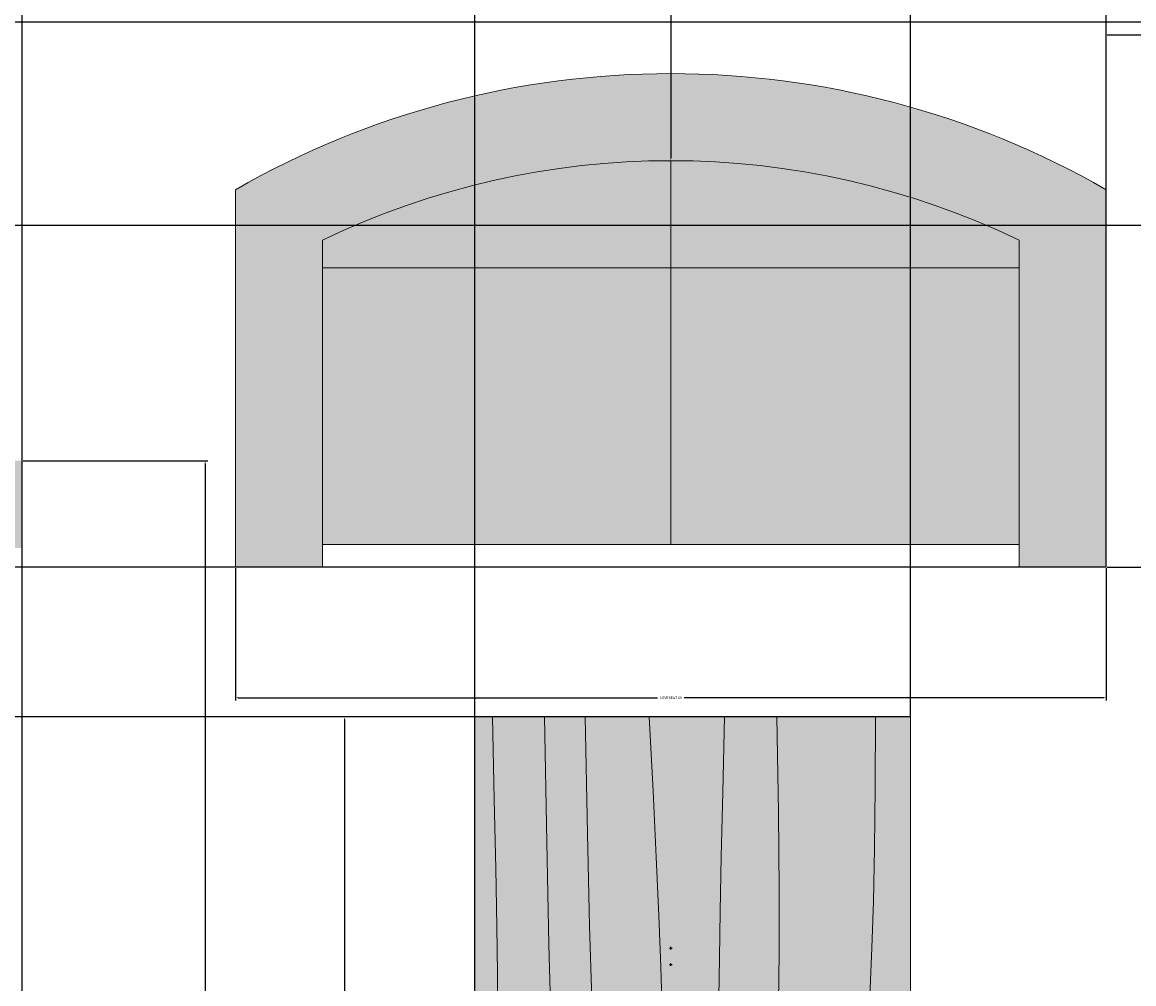
# Model space of a CAD drawing. Units: inches. Extents: x 1201 to 1754, y 247 to 775.
# Tile 4 of 10: x 1305 to 1382, y 491 to 557. Entities that reach past the tile are written whole.
import ezdxf

# ---------------------------------------------------------------- set-up
doc = ezdxf.new("R2010")
doc.units = ezdxf.units.IN
for name, color, linetype, lineweight in [('A-ANNO-DIMS', 2, 'Continuous', 18), ('A-FURN', 8, 'Continuous', 18), ('A-FURN-PATT', 9, 'Continuous', 13)]:
    doc.layers.add(name, color=color, linetype=linetype, lineweight=lineweight)
doc.styles.get("Standard").update_dxf_attribs({"font": 'arial.ttf'})
doc.dimstyles.get("Standard").update_dxf_attribs({"dimtxt": 0.18, "dimasz": 0.18, "dimexe": 0.18, "dimexo": 0.0625, "dimgap": 0.09, "dimtad": 0, "dimtih": 1, "dimtoh": 1, "dimdec": 4, "dimzin": 0, "dimdsep": 46, "dimtxsty": 'Standard', "dimcen": 0.09, "dimadec": 0, "dimazin": 0, "dimtfac": 1, "dimtdec": 4, "dimtofl": 0, "dimtmove": 0, "dimatfit": 3, "dimfxl": 1, "dimtolj": 1, "dimtzin": 0, "dimarcsym": 0})

# ---------------------------------------------------------------- blocks, each defined once
blk = doc.blocks.new('Sofa - Roundback Loveseat 5 ft.')
for p, q in [((0, -32.44198), (0, -5.99998)), ((-24, -33.99998), (-24, -11.46958)), ((24.00004, -33.99998), (24.00004, -11.46958)), ((-23.9998, -13.38178), (23.99986, -13.38178)), ((-24, -32.44198), (24.00004, -32.44198))]:
    blk.add_line(p, q)
for points in [[(-24, -33.99998), (-30, -33.99998), (-30, -7.99998)], [(30.00004, -7.99998), (30.00004, -33.99998), (24.00004, -33.99998)]]:
    blk.add_lwpolyline(points)
for centre, radius, start, end in [((0, -60.24998), 60.24998, 60.13715, 119.8628), ((0, -61.38438), 55.38444, 64.32083, 115.6792)]:
    blk.add_arc(centre, radius, start, end)
blk = doc.blocks.new('Table - Rectangular Woodgrain 60 x 30 in.')
for p, q in [((0, 0), (0, -30)), ((60, 0), (0, 0)), ((60, -30), (60, 0)), ((0, -30), (60, -30))]:
    blk.add_line(p, q)
for points in [[(0, -2.4), (4.8155, -2.418), (9.0302, -2.4688), (12.709, -2.5477), (15.9167, -2.65), (18.7181, -2.7711), (21.1781, -2.9063), (23.3616, -3.0508), (25.3333, -3.2), (27.1477, -3.3495), (28.8172, -3.4958), (30.3437, -3.636), (31.7291, -3.7667), (32.9756, -3.8849), (34.0849, -3.9875), (35.059, -4.0714), (35.9, -4.1334), (36.6114, -4.1711), (37.2041, -4.1854), (37.6906, -4.1779), (38.0833, -4.15), (38.3948, -4.1034), (38.6375, -4.0396), (38.8239, -3.9602), (38.9666, -3.8667), (39.0764, -3.7608), (39.1573, -3.6448), (39.2116, -3.521), (39.2416, -3.3917), (39.2498, -3.2593), (39.2385, -3.1261), (39.21, -2.9944), (39.1666, -2.8667), (39.111, -2.7447), (39.0468, -2.6281), (38.978, -2.5163), (38.9083, -2.4083), (38.8418, -2.3035), (38.7823, -2.201), (38.7337, -2.1001), (38.7, -2), (38.6844, -1.9003), (38.6875, -1.8021), (38.7094, -1.707), (38.75, -1.6167), (38.8094, -1.5326), (38.8875, -1.4563), (38.9844, -1.3893), (39.1, -1.3333), (39.2351, -1.2896), (39.3937, -1.2583), (39.5804, -1.2396), (39.8, -1.2333), (40.057, -1.2396), (40.3562, -1.2583), (40.7023, -1.2896), (41.1, -1.3333), (41.5547, -1.3895), (42.0755, -1.4573), (42.6721, -1.5361), (43.3542, -1.625), (44.1316, -1.7233), (45.014, -1.8302), (46.0114, -1.9449), (47.1333, -2.0667), (48.3862, -2.1947), (49.7625, -2.3281), (51.2513, -2.4663), (52.8416, -2.6083), (54.5226, -2.7535), (56.2833, -2.9011), (58.1127, -3.0501), (60, -3.2)], [(0, -9.2), (6.5759, -9.0858), (11.9385, -9.0365), (16.2527, -9.0418), (19.6833, -9.0917), (22.3952, -9.1759), (24.5531, -9.2844), (26.322, -9.4069), (27.8666, -9.5333), (29.3241, -9.6553), (30.7203, -9.7719), (32.0532, -9.8837), (33.3208, -9.9917), (34.5213, -10.0965), (35.6526, -10.199), (36.7128, -10.2999), (37.7, -10.4), (38.6129, -10.4996), (39.4531, -10.5969), (40.223, -10.6895), (40.925, -10.775), (41.5613, -10.8512), (42.1344, -10.9156), (42.6465, -10.966), (43.1, -11), (43.4976, -11.0158), (43.8437, -11.0136), (44.143, -10.9942), (44.4, -10.9583), (44.6195, -10.9069), (44.8062, -10.8406), (44.9648, -10.7603), (45.1, -10.6667), (45.2155, -10.5598), (45.3114, -10.4365), (45.3871, -10.2929), (45.4416, -10.125), (45.4743, -9.929), (45.4844, -9.7011), (45.4709, -9.4371), (45.4333, -9.1333), (45.3716, -8.7883), (45.2896, -8.4104), (45.1919, -8.0107), (45.0833, -7.6), (44.9685, -7.1893), (44.8521, -6.7896), (44.7388, -6.4117), (44.6333, -6.0667), (44.54, -5.7628), (44.4614, -5.4979), (44.4001, -5.2675), (44.3583, -5.0667), (44.3384, -4.8909), (44.3427, -4.7354), (44.3736, -4.5956), (44.4333, -4.4667), (44.5236, -4.3453), (44.6427, -4.2333), (44.7884, -4.1339), (44.9583, -4.05), (45.1501, -3.9849), (45.3614, -3.9417), (45.59, -3.9234), (45.8333, -3.9333), (46.0915, -3.9749), (46.3734, -4.0531), (46.6906, -4.1736), (47.0542, -4.3417), (47.4756, -4.5629), (47.9661, -4.8427), (48.5372, -5.1866), (49.2, -5.6), (49.9676, -6.0844), (50.8594, -6.625), (51.8965, -7.2031), (53.1, -7.8), (54.491, -8.3969), (56.0906, -8.975), (57.9199, -9.5156), (60, -10)], [(0, -12.8), (5.1847, -12.9322), (9.6213, -13.0323), (13.3963, -13.1059), (16.5958, -13.1583), (19.3063, -13.1952), (21.614, -13.2219), (23.6054, -13.2439), (25.3666, -13.2667), (26.9728, -13.2947), (28.4531, -13.3281), (29.8256, -13.3663), (31.1083, -13.4083), (32.3191, -13.4535), (33.476, -13.501), (34.597, -13.5501), (35.7, -13.6), (36.7984, -13.6497), (37.8875, -13.6979), (38.9578, -13.743), (40, -13.7833), (41.0047, -13.8174), (41.9625, -13.8438), (42.864, -13.8607), (43.7, -13.8667), (44.4631, -13.8604), (45.1552, -13.8417), (45.7801, -13.8104), (46.3416, -13.7667), (46.8439, -13.7104), (47.2906, -13.6417), (47.6858, -13.5604), (48.0333, -13.4667), (48.3375, -13.3608), (48.6042, -13.2448), (48.8396, -13.121), (49.05, -12.9917), (49.2417, -12.8593), (49.4208, -12.7261), (49.5937, -12.5944), (49.7667, -12.4667), (49.9452, -12.3451), (50.1323, -12.2313), (50.3303, -12.1268), (50.5416, -12.0333), (50.7686, -11.9524), (51.0135, -11.8854), (51.2788, -11.8341), (51.5666, -11.8), (51.8785, -11.7843), (52.2116, -11.7865), (52.562, -11.8059), (52.926, -11.8417), (53.2998, -11.8931), (53.6795, -11.9594), (54.0614, -12.0397), (54.4416, -12.1333), (54.8223, -12.2401), (55.2293, -12.3625), (55.6942, -12.5037), (56.2489, -12.6667), (56.9251, -12.8547), (57.7545, -13.0708), (58.7689, -13.3182), (60, -13.6)], [(0, -18), (5.124, -17.7273), (9.6609, -17.5057), (13.6705, -17.3303), (17.2125, -17.1958), (20.3467, -17.0973), (23.1328, -17.0297), (25.6307, -16.9878), (27.9, -16.9667), (29.9928, -16.9617), (31.9302, -16.9703), (33.7254, -16.9907), (35.3917, -17.0208), (36.9423, -17.0588), (38.3906, -17.1026), (39.7499, -17.1503), (41.0333, -17.2), (42.2519, -17.2496), (43.4073, -17.2969), (44.4986, -17.3395), (45.525, -17.375), (46.4858, -17.4012), (47.3802, -17.4156), (48.2074, -17.416), (48.9667, -17.4), (49.6583, -17.3662), (50.2872, -17.3167), (50.8595, -17.2547), (51.3812, -17.1833), (51.8584, -17.1057), (52.2971, -17.025), (52.7034, -16.9443), (53.0833, -16.8667), (53.443, -16.7951), (53.789, -16.7313), (54.128, -16.6768), (54.4666, -16.6334), (54.8115, -16.6024), (55.1693, -16.5854), (55.5465, -16.5841), (55.95, -16.6), (56.3828, -16.6337), (56.8346, -16.6823), (57.2915, -16.7418), (57.7396, -16.8084), (58.165, -16.878), (58.5539, -16.9469), (58.8924, -17.0111), (59.1666, -17.0667), (59.3679, -17.1107), (59.5078, -17.1438), (59.6032, -17.1675), (59.6708, -17.1833), (59.7275, -17.193), (59.7901, -17.1979), (59.8753, -17.1998), (60, -17.2)], [(0, -22.4), (8.0098, -22.2501), (14.4094, -22.1011), (19.4168, -21.9535), (23.25, -21.8083), (26.1269, -21.6663), (28.2656, -21.5281), (29.884, -21.3947), (31.2, -21.2667), (32.3967, -21.1448), (33.5172, -21.0292), (34.5697, -20.9198), (35.5625, -20.8167), (36.5037, -20.7198), (37.4015, -20.6292), (38.2642, -20.5448), (39.1, -20.4667), (39.9164, -20.3951), (40.7187, -20.3313), (41.5117, -20.2768), (42.3, -20.2333), (43.0883, -20.2024), (43.8812, -20.1854), (44.6836, -20.1841), (45.5, -20.2), (46.3328, -20.234), (47.1747, -20.2844), (48.0163, -20.3488), (48.8479, -20.425), (49.66, -20.5106), (50.4429, -20.6031), (51.1872, -20.7004), (51.8833, -20.8), (52.5246, -20.8999), (53.1166, -20.9995), (53.6681, -21.0983), (54.1875, -21.1958), (54.6834, -21.2919), (55.1646, -21.3859), (55.6394, -21.4777), (56.1167, -21.5667), (56.6028, -21.6515), (57.0961, -21.7266), (57.5929, -21.7852), (58.0896, -21.8208), (58.5823, -21.8268), (59.0674, -21.7964), (59.5412, -21.723), (60, -21.6)], [(0, -25.2), (8.6355, -25.0504), (15.7026, -24.9031), (21.4049, -24.7606), (25.9458, -24.625), (29.529, -24.4988), (32.3578, -24.3844), (34.6359, -24.284), (36.5667, -24.2), (38.3213, -24.1341), (39.9417, -24.0854), (41.437, -24.0523), (42.8167, -24.0333), (44.0901, -24.0268), (45.2667, -24.0313), (46.3557, -24.0451), (47.3667, -24.0667), (48.309, -24.0947), (49.1928, -24.1287), (50.0284, -24.168), (50.826, -24.2125), (51.5959, -24.2617), (52.3483, -24.3151), (53.0935, -24.3725), (53.8417, -24.4334), (54.6009, -24.497), (55.3699, -24.561), (56.1454, -24.6226), (56.9239, -24.6792), (57.7021, -24.7279), (58.4764, -24.7662), (59.2435, -24.7911), (60, -24.8)], [(0, -28.8), (5.6867, -28.6681), (10.45, -28.5698), (14.407, -28.5012), (17.675, -28.4584), (20.3711, -28.4374), (22.6125, -28.4344), (24.5164, -28.4455), (26.2, -28.4667), (27.762, -28.4947), (29.2276, -28.5281), (30.6033, -28.5663), (31.8958, -28.6084), (33.1118, -28.6535), (34.2578, -28.7011), (35.3405, -28.7501), (36.3666, -28.8), (37.3443, -28.8497), (38.288, -28.8974), (39.2137, -28.9412), (40.1375, -28.9792), (41.0753, -29.0093), (42.0432, -29.0297), (43.0572, -29.0384), (44.1333, -29.0333), (45.2936, -29.0114), (46.5843, -28.9641), (48.0579, -28.8816), (49.7666, -28.7542), (51.7629, -28.5721), (54.0989, -28.3255), (56.8272, -28.0048), (60, -27.6)]]:
    blk.add_lwpolyline(points)
blk = doc.blocks.new('*D31')
at = {"layer": 'A-ANNO-DIMS', "color": 0, "lineweight": -2, "transparency": 16777216}
for p, q in [((1319.706, 519.841), (1319.706, 510.723)), ((1379.706, 519.841), (1379.706, 510.723)), ((1319.886, 510.903), (1348.792, 510.903)), ((1379.526, 510.903), (1350.619, 510.903))]:
    blk.add_line(p, q, dxfattribs=at)
at = {"layer": 'A-ANNO-DIMS', "color": 0, "transparency": 16777216}
for points in [[(1319.886, 510.933), (1319.886, 510.873), (1319.706, 510.903)], [(1379.526, 510.933), (1379.526, 510.873), (1379.706, 510.903)]]:
    blk.add_solid(points, dxfattribs=at)
at = {"layer": 'Defpoints', "color": 0, "transparency": 16777216}
for p in [(1319.706, 519.903), (1379.706, 519.903), (1379.706, 510.903)]:
    blk.add_point(p, dxfattribs=at)
at = {"layer": 'A-ANNO-DIMS', "color": 0, "transparency": 16777216, "insert": (1349.706, 510.903), "char_height": 0.18, "attachment_point": 5}
blk.add_mtext('\\A1;LOVESEAT 60', dxfattribs=at)
blk = doc.blocks.new('*D32')
at = {"layer": 'A-ANNO-DIMS', "color": 0, "lineweight": -2, "transparency": 16777216}
for p, q in [((1379.768, 556.57), (1388.886, 556.57)), ((1388.706, 556.39), (1388.706, 538.419)), ((1388.706, 520.083), (1388.706, 538.055)), ((1379.768, 519.903), (1388.886, 519.903))]:
    blk.add_line(p, q, dxfattribs=at)
at = {"layer": 'A-ANNO-DIMS', "color": 0, "transparency": 16777216}
for points in [[(1388.676, 556.39), (1388.736, 556.39), (1388.706, 556.57)], [(1388.676, 520.083), (1388.736, 520.083), (1388.706, 519.903)]]:
    blk.add_solid(points, dxfattribs=at)
at = {"layer": 'Defpoints', "color": 0, "transparency": 16777216}
for p in [(1379.706, 556.57), (1388.706, 556.57), (1379.706, 519.903)]:
    blk.add_point(p, dxfattribs=at)
at = {"layer": 'A-ANNO-DIMS', "color": 0, "transparency": 16777216, "insert": (1388.706, 538.237), "char_height": 0.18, "attachment_point": 5}
blk.add_mtext('\\A1;37', dxfattribs=at)
blk = doc.blocks.new('*D35')
at = {"layer": 'A-ANNO-DIMS', "color": 0, "lineweight": -2, "transparency": 16777216}
for p, q in [((1336.149, 509.584), (1327.031, 509.584)), ((1327.211, 509.404), (1327.211, 479.767)), ((1327.211, 449.764), (1327.211, 479.401)), ((1336.149, 449.584), (1327.031, 449.584))]:
    blk.add_line(p, q, dxfattribs=at)
at = {"layer": 'A-ANNO-DIMS', "color": 0, "transparency": 16777216}
for points in [[(1327.181, 509.404), (1327.241, 509.404), (1327.211, 509.584)], [(1327.181, 449.764), (1327.241, 449.764), (1327.211, 449.584)]]:
    blk.add_solid(points, dxfattribs=at)
at = {"layer": 'Defpoints', "color": 0, "transparency": 16777216}
for p in [(1336.211, 509.584), (1327.211, 449.584), (1336.211, 449.584)]:
    blk.add_point(p, dxfattribs=at)
at = {"layer": 'A-ANNO-DIMS', "color": 0, "transparency": 16777216, "insert": (1327.211, 479.584), "char_height": 0.18, "attachment_point": 5}
blk.add_mtext('\\A1;COFFEE TABLE 60', dxfattribs=at)
blk = doc.blocks.new('*D37')
at = {"layer": 'A-ANNO-DIMS', "color": 0, "lineweight": -2, "transparency": 16777216}
for p, q in [((1305.079, 527.227), (1317.797, 527.227)), ((1317.617, 527.047), (1317.617, 485.41)), ((1317.617, 443.407), (1317.617, 485.044)), ((1305.079, 443.227), (1317.797, 443.227))]:
    blk.add_line(p, q, dxfattribs=at)
at = {"layer": 'A-ANNO-DIMS', "color": 0, "transparency": 16777216}
for points in [[(1317.587, 527.047), (1317.647, 527.047), (1317.617, 527.227)], [(1317.587, 443.407), (1317.647, 443.407), (1317.617, 443.227)]]:
    blk.add_solid(points, dxfattribs=at)
at = {"layer": 'Defpoints', "color": 0, "transparency": 16777216}
for p in [(1305.017, 527.227), (1317.617, 527.227), (1305.017, 443.227)]:
    blk.add_point(p, dxfattribs=at)
at = {"layer": 'A-ANNO-DIMS', "color": 0, "transparency": 16777216, "insert": (1317.617, 485.227), "char_height": 0.18, "attachment_point": 5}
blk.add_mtext('\\A1;SOFA 84', dxfattribs=at)
blk = doc.blocks.new('*D59')
at = {"layer": 'A-ANNO-DIMS', "color": 0, "lineweight": -2, "transparency": 16777216}
for p, q in [((1255.521, 418.004), (1255.521, 775.136)), ((1405.521, 418.004), (1405.521, 775.136)), ((1255.701, 774.956), (1330.241, 774.956)), ((1405.341, 774.956), (1330.801, 774.956))]:
    blk.add_line(p, q, dxfattribs=at)
at = {"layer": 'A-ANNO-DIMS', "color": 0, "transparency": 16777216}
for points in [[(1255.701, 774.986), (1255.701, 774.926), (1255.521, 774.956)], [(1405.341, 774.986), (1405.341, 774.926), (1405.521, 774.956)]]:
    blk.add_solid(points, dxfattribs=at)
at = {"layer": 'Defpoints', "color": 0, "transparency": 16777216}
for p in [(1405.521, 774.956), (1255.521, 417.941), (1405.521, 417.941)]:
    blk.add_point(p, dxfattribs=at)
at = {"layer": 'A-ANNO-DIMS', "color": 0, "transparency": 16777216, "insert": (1330.521, 774.956), "char_height": 0.18, "attachment_point": 5}
blk.add_mtext('\\A1;150', dxfattribs=at)
blk = doc.blocks.new('*D75')
at = {"layer": 'A-ANNO-DIMS', "color": 0, "lineweight": -2, "transparency": 16777216}
for p, q in [((1717.458, 557.441), (1222.326, 557.441)), ((1222.506, 557.261), (1222.506, 550.621)), ((1222.506, 543.616), (1222.506, 550.257)), ((1717.458, 543.436), (1222.326, 543.436))]:
    blk.add_line(p, q, dxfattribs=at)
at = {"layer": 'A-ANNO-DIMS', "color": 0, "transparency": 16777216}
for points in [[(1222.476, 557.261), (1222.536, 557.261), (1222.506, 557.441)], [(1222.476, 543.616), (1222.536, 543.616), (1222.506, 543.436)]]:
    blk.add_solid(points, dxfattribs=at)
at = {"layer": 'Defpoints', "color": 0, "transparency": 16777216}
for p in [(1222.506, 557.441), (1717.521, 557.441), (1717.521, 543.436)]:
    blk.add_point(p, dxfattribs=at)
at = {"layer": 'A-ANNO-DIMS', "color": 0, "transparency": 16777216, "insert": (1222.506, 550.439), "char_height": 0.18, "attachment_point": 5}
blk.add_mtext('\\A1;14.005', dxfattribs=at)
blk = doc.blocks.new('*D83')
at = {"layer": 'A-ANNO-DIMS', "color": 0, "lineweight": -2, "transparency": 16777216}
for p, q in [((1471.458, 561.969), (1222.326, 561.969)), ((1222.506, 561.789), (1222.506, 559.887)), ((1222.506, 557.621), (1222.506, 559.523)), ((1471.458, 557.441), (1222.326, 557.441))]:
    blk.add_line(p, q, dxfattribs=at)
at = {"layer": 'A-ANNO-DIMS', "color": 0, "transparency": 16777216}
for points in [[(1222.476, 561.789), (1222.536, 561.789), (1222.506, 561.969)], [(1222.476, 557.621), (1222.536, 557.621), (1222.506, 557.441)]]:
    blk.add_solid(points, dxfattribs=at)
at = {"layer": 'Defpoints', "color": 0, "transparency": 16777216}
for p in [(1222.506, 561.969), (1471.521, 561.969), (1471.521, 557.441)]:
    blk.add_point(p, dxfattribs=at)
at = {"layer": 'A-ANNO-DIMS', "color": 0, "transparency": 16777216, "insert": (1222.506, 559.705), "char_height": 0.18, "attachment_point": 5}
blk.add_mtext('\\A1;4.528', dxfattribs=at)
blk = doc.blocks.new('*D94')
at = {"layer": 'A-ANNO-DIMS', "color": 0, "lineweight": -2, "transparency": 16777216}
for p, q in [((1305.017, 443.289), (1305.017, 775.136)), ((1336.211, 449.646), (1336.211, 775.136)), ((1305.197, 774.956), (1320.15, 774.956)), ((1336.031, 774.956), (1321.078, 774.956))]:
    blk.add_line(p, q, dxfattribs=at)
at = {"layer": 'A-ANNO-DIMS', "color": 0, "transparency": 16777216}
for points in [[(1305.197, 774.986), (1305.197, 774.926), (1305.017, 774.956)], [(1336.031, 774.986), (1336.031, 774.926), (1336.211, 774.956)]]:
    blk.add_solid(points, dxfattribs=at)
at = {"layer": 'Defpoints', "color": 0, "transparency": 16777216}
for p in [(1336.211, 774.956), (1336.211, 449.584), (1305.017, 443.227)]:
    blk.add_point(p, dxfattribs=at)
at = {"layer": 'A-ANNO-DIMS', "color": 0, "transparency": 16777216, "insert": (1320.614, 774.956), "char_height": 0.18, "attachment_point": 5}
blk.add_mtext('\\A1;31.195', dxfattribs=at)
blk = doc.blocks.new('*D98')
at = {"layer": 'A-ANNO-DIMS', "color": 0, "lineweight": -2, "transparency": 16777216}
for p, q in [((1366.211, 509.646), (1366.211, 775.136)), ((1379.706, 519.966), (1379.706, 775.136)), ((1366.391, 774.956), (1372.504, 774.956)), ((1379.526, 774.956), (1373.413, 774.956))]:
    blk.add_line(p, q, dxfattribs=at)
at = {"layer": 'A-ANNO-DIMS', "color": 0, "transparency": 16777216}
for points in [[(1366.391, 774.986), (1366.391, 774.926), (1366.211, 774.956)], [(1379.526, 774.986), (1379.526, 774.926), (1379.706, 774.956)]]:
    blk.add_solid(points, dxfattribs=at)
at = {"layer": 'Defpoints', "color": 0, "transparency": 16777216}
for p in [(1379.706, 774.956), (1379.706, 519.903), (1366.211, 509.584)]:
    blk.add_point(p, dxfattribs=at)
at = {"layer": 'A-ANNO-DIMS', "color": 0, "transparency": 16777216, "insert": (1372.959, 774.956), "char_height": 0.18, "attachment_point": 5}
blk.add_mtext('\\A1;13.494', dxfattribs=at)
blk = doc.blocks.new('*D99')
at = {"layer": 'A-ANNO-DIMS', "color": 0, "lineweight": -2, "transparency": 16777216}
for p, q in [((1379.643, 519.903), (1222.326, 519.903)), ((1222.506, 519.723), (1222.506, 514.926)), ((1222.506, 509.764), (1222.506, 514.562)), ((1366.149, 509.584), (1222.326, 509.584))]:
    blk.add_line(p, q, dxfattribs=at)
at = {"layer": 'A-ANNO-DIMS', "color": 0, "transparency": 16777216}
for points in [[(1222.476, 519.723), (1222.536, 519.723), (1222.506, 519.903)], [(1222.476, 509.764), (1222.536, 509.764), (1222.506, 509.584)]]:
    blk.add_solid(points, dxfattribs=at)
at = {"layer": 'Defpoints', "color": 0, "transparency": 16777216}
for p in [(1222.506, 519.903), (1379.706, 519.903), (1366.211, 509.584)]:
    blk.add_point(p, dxfattribs=at)
at = {"layer": 'A-ANNO-DIMS', "color": 0, "transparency": 16777216, "insert": (1222.506, 514.744), "char_height": 0.18, "attachment_point": 5}
blk.add_mtext('\\A1;10.32', dxfattribs=at)
blk = doc.blocks.new('*D103')
at = {"layer": 'A-ANNO-DIMS', "color": 0, "lineweight": -2, "transparency": 16777216}
for p, q in [((1349.886, 590.053), (1349.706, 590.053)), ((1349.706, 590.053), (1349.706, 554.083)), ((1349.616, 493.653), (1349.796, 493.653)), ((1349.706, 493.563), (1349.706, 493.743))]:
    blk.add_line(p, q, dxfattribs=at)
at = {"layer": 'A-ANNO-DIMS', "color": 0, "transparency": 16777216}
blk.add_solid([(1349.676, 554.083), (1349.736, 554.083), (1349.706, 553.903)], dxfattribs=at)
at = {"layer": 'Defpoints', "color": 0, "transparency": 16777216}
for p in [(1349.706, 553.903), (1349.706, 493.653)]:
    blk.add_point(p, dxfattribs=at)
at = {"layer": 'A-ANNO-DIMS', "color": 0, "transparency": 16777216, "insert": (1350.367, 590.053), "char_height": 0.18, "attachment_point": 5}
blk.add_mtext('\\A1;R60.25', dxfattribs=at)
blk = doc.blocks.new('*D104')
at = {"layer": 'A-ANNO-DIMS', "color": 0, "lineweight": -2, "transparency": 16777216}
for p, q in [((1349.886, 581.134), (1349.706, 581.134)), ((1349.706, 581.134), (1349.706, 548.084)), ((1349.616, 492.519), (1349.796, 492.519)), ((1349.706, 492.429), (1349.706, 492.609))]:
    blk.add_line(p, q, dxfattribs=at)
at = {"layer": 'A-ANNO-DIMS', "color": 0, "transparency": 16777216}
blk.add_solid([(1349.676, 548.084), (1349.736, 548.084), (1349.706, 547.904)], dxfattribs=at)
at = {"layer": 'Defpoints', "color": 0, "transparency": 16777216}
for p in [(1349.706, 547.904), (1349.706, 492.519)]:
    blk.add_point(p, dxfattribs=at)
at = {"layer": 'A-ANNO-DIMS', "color": 0, "transparency": 16777216, "insert": (1350.366, 581.134), "char_height": 0.18, "attachment_point": 5}
blk.add_mtext('\\A1;R55.38', dxfattribs=at)

msp = doc.modelspace()

# ---------------------------------------------------------------- hatches: boundary and pattern name
at = {"layer": 'A-FURN-PATT'}
h = msp.add_hatch(color=256, dxfattribs=at)
h.dxf.hatch_style = 1
h.paths.add_polyline_path([(1373.7057, 540.5217), (1349.7056, 540.5217), (1349.7056, 521.4615), (1373.7057, 521.4615)], flags=17)
h.paths.add_polyline_path([(1349.7056, 540.5217), (1325.7056, 540.5217), (1325.7056, 521.4615), (1349.7056, 521.4615)], flags=17)
h.paths.add_polyline_path([(1349.7056, 547.9035, 0.1125187), (1325.7056, 542.4334), (1325.7056, 540.5217), (1349.7056, 540.5217)], flags=17)
h.paths.add_polyline_path([(1349.7056, 547.9035), (1349.7056, 540.5217), (1373.7057, 540.5217), (1373.7057, 542.4333, 0.1125189)], flags=17)
h.paths.add_polyline_path([(1319.7056, 545.9034), (1319.7056, 519.9035), (1325.7056, 519.9035), (1325.7056, 542.4334, -0.2279232), (1373.7057, 542.4333), (1373.7057, 540.5217), (1373.7057, 521.4615), (1373.7057, 519.9035), (1379.7057, 519.9035), (1379.7057, 545.9034, 0.266667)])
h.paths.add_polyline_path([(1303.4586, 521.2267), (1284.3984, 521.2267), (1284.3984, 497.2267), (1303.4586, 497.2267)], flags=17)
h.paths.add_polyline_path([(1303.4586, 497.2267), (1284.3984, 497.2267), (1284.3984, 473.2267), (1303.4586, 473.2267)], flags=17)
h.paths.add_polyline_path([(1303.4586, 473.2267), (1284.3984, 473.2267), (1284.3984, 449.2267), (1303.4586, 449.2267)], flags=17)
h.paths.add_polyline_path([(1282.4866, 521.2267), (1305.0165, 521.2267), (1305.0165, 527.2267), (1279.0165, 527.2267, 0.1904762), (1279.0165, 443.2267), (1305.0165, 443.2267), (1305.0165, 449.2267), (1282.4866, 449.2267, -0.1519478)])
h.paths.add_polyline_path([(1284.3984, 497.2267), (1277.612, 497.2267, 0.0496282), (1277.612, 473.2267), (1284.3984, 473.2267)], flags=17)
h.paths.add_polyline_path([(1284.3984, 521.2267), (1282.4866, 521.2267, 0.0506467), (1277.612, 497.2267), (1284.3984, 497.2267)], flags=17)
h.paths.add_polyline_path([(1284.3984, 473.2267), (1277.612, 473.2267, 0.0506466), (1282.4866, 449.2267), (1284.3984, 449.2267)], flags=17)
h = msp.add_hatch(color=256, dxfattribs=at)
h.dxf.hatch_style = 1
h.paths.add_polyline_path([(1363.7933, 504.7684), (1363.8113, 509.5839), (1357.0113, 509.5839), (1357.1255, 503.008), (1357.1748, 497.6454), (1357.1695, 493.3312), (1357.1196, 489.9006), (1357.0354, 487.1887), (1356.9269, 485.0308), (1356.8044, 483.2619), (1356.678, 481.7173), (1356.556, 480.2598), (1356.4394, 478.8636), (1356.3276, 477.5307), (1356.2196, 476.2631), (1356.1148, 475.0626), (1356.0123, 473.9313), (1355.9114, 472.8711), (1355.8113, 471.8839), (1355.7117, 470.971), (1355.6144, 470.1308), (1355.5218, 469.3609), (1355.4363, 468.6589), (1355.3601, 468.0226), (1355.2957, 467.4495), (1355.2453, 466.9374), (1355.2113, 466.4839), (1355.1955, 466.0863), (1355.1977, 465.7402), (1355.2171, 465.4409), (1355.253, 465.1839), (1355.3044, 464.9644), (1355.3707, 464.7777), (1355.451, 464.6191), (1355.5446, 464.4839), (1355.6515, 464.3684), (1355.7748, 464.2725), (1355.9184, 464.1968), (1356.0863, 464.1423), (1356.2823, 464.1096), (1356.5102, 464.0995), (1356.7742, 464.113), (1357.078, 464.1506), (1357.423, 464.2123), (1357.8009, 464.2943), (1358.2006, 464.392), (1358.6113, 464.5006), (1359.022, 464.6154), (1359.4217, 464.7318), (1359.7996, 464.8451), (1360.1446, 464.9506), (1360.4485, 465.0439), (1360.7134, 465.1225), (1360.9438, 465.1838), (1361.1446, 465.2256), (1361.3204, 465.2455), (1361.4759, 465.2412), (1361.6157, 465.2103), (1361.7446, 465.1506), (1361.866, 465.0603), (1361.978, 464.9412), (1362.0774, 464.7955), (1362.1613, 464.6256), (1362.2264, 464.4338), (1362.2696, 464.2225), (1362.2879, 463.9939), (1362.278, 463.7506), (1362.2364, 463.4924), (1362.1582, 463.2105), (1362.0377, 462.8933), (1361.8696, 462.5297), (1361.6484, 462.1083), (1361.3686, 461.6178), (1361.0247, 461.0467), (1360.6113, 460.3839), (1360.1269, 459.6163), (1359.5863, 458.7245), (1359.0082, 457.6874), (1358.4113, 456.4839), (1357.8144, 455.0929), (1357.2363, 453.4933), (1356.6957, 451.664), (1356.2113, 449.5839), (1363.0113, 449.5839), (1363.1612, 451.4712), (1363.3102, 453.3006), (1363.4578, 455.0613), (1363.603, 456.7423), (1363.745, 458.3326), (1363.8832, 459.8214), (1364.0166, 461.1977), (1364.1446, 462.4506), (1364.2664, 463.5725), (1364.3811, 464.5699), (1364.488, 465.4523), (1364.5863, 466.2297), (1364.6752, 466.9118), (1364.754, 467.5084), (1364.8218, 468.0292), (1364.878, 468.4839), (1364.9217, 468.8816), (1364.953, 469.2277), (1364.9717, 469.5269), (1364.978, 469.7839), (1364.9717, 470.0035), (1364.953, 470.1902), (1364.9217, 470.3488), (1364.878, 470.4839), (1364.822, 470.5995), (1364.755, 470.6964), (1364.6787, 470.7745), (1364.5946, 470.8339), (1364.5043, 470.8745), (1364.4092, 470.8964), (1364.311, 470.8995), (1364.2113, 470.8839), (1364.1112, 470.8502), (1364.0103, 470.8016), (1363.9078, 470.7421), (1363.803, 470.6756), (1363.6186, 470.5566), (1363.3995, 470.436), (1363.149, 470.3508), (1362.881, 470.3281), (1362.6903, 470.3723), (1362.5665, 470.4266), (1362.4505, 470.5075), (1362.3446, 470.6173), (1362.2511, 470.76), (1362.1717, 470.9464), (1362.1079, 471.1891), (1362.0613, 471.5006), (1362.0334, 471.8933), (1362.0259, 472.3798), (1362.0402, 472.9725), (1362.0779, 473.6839), (1362.1399, 474.5249), (1362.2238, 475.499), (1362.3264, 476.6083), (1362.4446, 477.8548), (1362.5753, 479.2402), (1362.7155, 480.7667), (1362.8618, 482.4362), (1363.0113, 484.2506), (1363.1605, 486.2223), (1363.305, 488.4058), (1363.4402, 490.8658), (1363.5613, 493.6672), (1363.6636, 496.8749), (1363.7425, 500.5537)])
h.paths.add_polyline_path([(1342.1259, 469.6422), (1342.0772, 471.2626), (1342.0113, 473.0172), (1341.9273, 474.948), (1341.8269, 477.2261), (1341.7125, 480.0549), (1341.5863, 483.6381), (1341.4507, 488.179), (1341.3082, 493.8813), (1341.1609, 500.9484), (1341.0113, 509.5839), (1337.4113, 509.5839), (1337.5432, 503.8972), (1337.6415, 499.1339), (1337.7101, 495.1769), (1337.7529, 491.9089), (1337.7739, 489.2128), (1337.7769, 486.9714), (1337.7658, 485.0675), (1337.7446, 483.3839), (1337.7166, 481.8219), (1337.6832, 480.3563), (1337.645, 478.9806), (1337.6029, 477.6881), (1337.5578, 476.4721), (1337.5102, 475.3261), (1337.4612, 474.2434), (1337.4113, 473.2173), (1337.3616, 472.2396), (1337.3139, 471.2959), (1337.2701, 470.3702), (1337.2321, 469.4464), (1337.202, 468.5086), (1337.1816, 467.5407), (1337.1729, 466.5267), (1337.178, 465.4506), (1337.1999, 464.2903), (1337.2472, 462.9996), (1337.3297, 461.526), (1337.4571, 459.8173), (1337.6392, 457.821), (1337.8858, 455.485), (1338.2065, 452.7567), (1338.6113, 449.5839), (1341.4113, 449.5839), (1341.4202, 450.3404), (1341.4451, 451.1075), (1341.4834, 451.8818), (1341.5321, 452.66), (1341.5887, 453.4385), (1341.6503, 454.214), (1341.7143, 454.983), (1341.7779, 455.7422), (1341.8388, 456.4904), (1341.8962, 457.2356), (1341.9496, 457.988), (1341.9988, 458.7579), (1342.0433, 459.5555), (1342.0826, 460.3911), (1342.1166, 461.2749), (1342.1446, 462.2172), (1342.1662, 463.2282), (1342.18, 464.3172), (1342.1845, 465.4938), (1342.178, 466.7672), (1342.159, 468.1469)])
h.paths.add_polyline_path([(1345.8625, 461.5676), (1345.9269, 462.4092), (1345.9773, 463.2511), (1346.0113, 464.0839), (1346.0272, 464.9003), (1346.0259, 465.7027), (1346.0089, 466.4956), (1345.978, 467.2839), (1345.9345, 468.0722), (1345.88, 468.8652), (1345.8162, 469.6675), (1345.7446, 470.4839), (1345.6665, 471.3197), (1345.5821, 472.1824), (1345.4915, 473.0802), (1345.3946, 474.0214), (1345.2915, 475.0142), (1345.1821, 476.0667), (1345.0665, 477.1872), (1344.9446, 478.3839), (1344.8166, 479.6999), (1344.6832, 481.3183), (1344.545, 483.457), (1344.403, 486.3339), (1344.2578, 490.1671), (1344.1102, 495.1745), (1343.9612, 501.5741), (1343.8113, 509.5839), (1341.0113, 509.5839), (1341.1609, 500.9484), (1341.3082, 493.8813), (1341.4507, 488.179), (1341.5863, 483.6381), (1341.7125, 480.0549), (1341.8269, 477.2261), (1341.9273, 474.948), (1342.0113, 473.0172), (1342.0772, 471.2626), (1342.1259, 469.6422), (1342.159, 468.1469), (1342.178, 466.7672), (1342.1845, 465.4938), (1342.18, 464.3172), (1342.1662, 463.2282), (1342.1446, 462.2172), (1342.1166, 461.2749), (1342.0826, 460.3911), (1342.0433, 459.5555), (1341.9988, 458.7579), (1341.9496, 457.988), (1341.8962, 457.2356), (1341.8388, 456.4904), (1341.7779, 455.7422), (1341.7143, 454.983), (1341.6503, 454.214), (1341.5887, 453.4385), (1341.5321, 452.66), (1341.4834, 451.8818), (1341.4451, 451.1075), (1341.4202, 450.3404), (1341.4113, 449.5839), (1344.6113, 449.5839), (1344.4883, 450.0427), (1344.4149, 450.5165), (1344.3845, 451.0016), (1344.3905, 451.4943), (1344.4261, 451.991), (1344.4847, 452.4878), (1344.5598, 452.9811), (1344.6446, 453.4672), (1344.7336, 453.9445), (1344.8254, 454.4193), (1344.9194, 454.9005), (1345.0155, 455.3964), (1345.113, 455.9158), (1345.2118, 456.4673), (1345.3114, 457.0593), (1345.4113, 457.7006), (1345.5109, 458.3967), (1345.6082, 459.141), (1345.7007, 459.9239), (1345.7863, 460.736)])
h.paths.add_polyline_path([(1349.1056, 457.7255), (1349.028, 458.2027), (1348.9566, 458.7244), (1348.8946, 459.2967), (1348.8451, 459.9256), (1348.8113, 460.6172), (1348.7953, 461.3765), (1348.7957, 462.2037), (1348.8101, 463.0981), (1348.8363, 464.0589), (1348.8718, 465.0853), (1348.9144, 466.1766), (1348.9617, 467.332), (1349.0113, 468.5506), (1349.061, 469.834), (1349.1087, 471.1933), (1349.1525, 472.6416), (1349.1905, 474.1922), (1349.2206, 475.8585), (1349.241, 477.6537), (1349.2496, 479.5911), (1349.2446, 481.6839), (1349.2235, 483.9532), (1349.1816, 486.4511), (1349.114, 489.2372), (1349.0155, 492.3714), (1348.881, 495.9134), (1348.7056, 499.923), (1348.484, 504.4599), (1348.2113, 509.5839), (1343.8113, 509.5839), (1343.9612, 501.5741), (1344.1102, 495.1745), (1344.2578, 490.1671), (1344.403, 486.3339), (1344.545, 483.457), (1344.6832, 481.3183), (1344.8166, 479.6999), (1344.9446, 478.3839), (1345.0665, 477.1872), (1345.1821, 476.0667), (1345.2915, 475.0142), (1345.3946, 474.0214), (1345.4915, 473.0802), (1345.5821, 472.1824), (1345.6665, 471.3197), (1345.7446, 470.4839), (1345.8162, 469.6675), (1345.88, 468.8652), (1345.9345, 468.0722), (1345.978, 467.2839), (1346.0089, 466.4956), (1346.0259, 465.7027), (1346.0272, 464.9003), (1346.0113, 464.0839), (1345.9773, 463.2511), (1345.9269, 462.4092), (1345.8625, 461.5676), (1345.7863, 460.736), (1345.7007, 459.9239), (1345.6082, 459.141), (1345.5109, 458.3967), (1345.4113, 457.7006), (1345.3114, 457.0593), (1345.2118, 456.4673), (1345.113, 455.9158), (1345.0155, 455.3964), (1344.9194, 454.9005), (1344.8254, 454.4193), (1344.7336, 453.9445), (1344.6446, 453.4672), (1344.5598, 452.9811), (1344.4847, 452.4878), (1344.4261, 451.991), (1344.3905, 451.4943), (1344.3845, 451.0016), (1344.4149, 450.5165), (1344.4883, 450.0427), (1344.6113, 449.5839), (1349.0113, 449.5839), (1349.0117, 449.8177), (1349.0302, 449.9259), (1349.0675, 450.0761), (1349.1006, 450.216), (1349.1446, 450.4173), (1349.2002, 450.6915), (1349.2644, 451.03), (1349.3333, 451.4189), (1349.4029, 451.8443), (1349.4695, 452.2924), (1349.529, 452.7493), (1349.5776, 453.2011), (1349.6113, 453.6339), (1349.6272, 454.0374), (1349.6259, 454.4146), (1349.6089, 454.7724), (1349.5779, 455.1173), (1349.5345, 455.4559), (1349.48, 455.7949), (1349.4162, 456.1409), (1349.3446, 456.5006), (1349.267, 456.8805), (1349.1863, 457.2868)])
h.paths.add_polyline_path([(1354.4248, 457.3723), (1354.427, 457.7054), (1354.4113, 458.0173), (1354.3772, 458.3051), (1354.3259, 458.5704), (1354.2589, 458.8153), (1354.178, 459.0423), (1354.0845, 459.2536), (1353.98, 459.4516), (1353.8662, 459.6387), (1353.7446, 459.8172), (1353.6169, 459.9902), (1353.4852, 460.1631), (1353.352, 460.3422), (1353.2196, 460.5339), (1353.0903, 460.7443), (1352.9665, 460.9797), (1352.8505, 461.2464), (1352.7446, 461.5506), (1352.6509, 461.8981), (1352.5696, 462.2933), (1352.5009, 462.74), (1352.4446, 463.2423), (1352.4009, 463.8038), (1352.3696, 464.4287), (1352.3509, 465.1208), (1352.3446, 465.8839), (1352.3506, 466.7199), (1352.3675, 467.6214), (1352.3939, 468.5792), (1352.428, 469.5839), (1352.4683, 470.6261), (1352.5134, 471.6964), (1352.5616, 472.7855), (1352.6113, 473.8839), (1352.6612, 474.9869), (1352.7103, 476.1079), (1352.7578, 477.2648), (1352.803, 478.4756), (1352.845, 479.7583), (1352.8832, 481.1308), (1352.9166, 482.6111), (1352.9446, 484.2173), (1352.9674, 485.9785), (1352.9894, 487.9699), (1353.0161, 490.2776), (1353.053, 492.9881), (1353.1054, 496.1876), (1353.179, 499.9626), (1353.2791, 504.3992), (1353.4113, 509.5839), (1348.2113, 509.5839), (1348.484, 504.4599), (1348.7056, 499.923), (1348.881, 495.9134), (1349.0155, 492.3714), (1349.114, 489.2372), (1349.1816, 486.4511), (1349.2235, 483.9532), (1349.2446, 481.6839), (1349.2496, 479.5911), (1349.241, 477.6537), (1349.2206, 475.8585), (1349.1905, 474.1922), (1349.1525, 472.6416), (1349.1087, 471.1933), (1349.061, 469.834), (1349.0113, 468.5506), (1348.9617, 467.332), (1348.9144, 466.1766), (1348.8718, 465.0853), (1348.8363, 464.0589), (1348.8101, 463.0981), (1348.7957, 462.2037), (1348.7953, 461.3765), (1348.8113, 460.6172), (1348.8451, 459.9256), (1348.8946, 459.2967), (1348.9566, 458.7244), (1349.028, 458.2027), (1349.1056, 457.7255), (1349.1863, 457.2868), (1349.267, 456.8805), (1349.3446, 456.5006), (1349.4162, 456.1409), (1349.48, 455.7949), (1349.5345, 455.4559), (1349.5779, 455.1173), (1349.6089, 454.7724), (1349.6259, 454.4146), (1349.6272, 454.0374), (1349.6113, 453.6339), (1349.5776, 453.2011), (1349.529, 452.7493), (1349.4695, 452.2924), (1349.4029, 451.8443), (1349.3333, 451.4189), (1349.2644, 451.03), (1349.2002, 450.6915), (1349.1446, 450.4173), (1349.1006, 450.216), (1349.0675, 450.0761), (1349.0438, 449.9807), (1349.028, 449.9131), (1349.0183, 449.8564), (1349.0134, 449.7938), (1349.0115, 449.7086), (1349.0113, 449.5839), (1352.6113, 449.5839), (1352.8931, 450.815), (1353.1405, 451.8294), (1353.3566, 452.6588), (1353.5446, 453.335), (1353.7076, 453.8897), (1353.8488, 454.3546), (1353.9712, 454.7616), (1354.078, 455.1423), (1354.1716, 455.5225), (1354.2519, 455.9044), (1354.3182, 456.2841), (1354.3696, 456.6579), (1354.4054, 457.0219)])
h.paths.add_polyline_path([(1360.1269, 459.6163), (1360.6113, 460.3839), (1361.0247, 461.0467), (1361.3686, 461.6178), (1361.6484, 462.1083), (1361.8696, 462.5297), (1362.0377, 462.8933), (1362.1582, 463.2105), (1362.2364, 463.4924), (1362.278, 463.7506), (1362.2879, 463.9939), (1362.2696, 464.2225), (1362.2264, 464.4338), (1362.1613, 464.6256), (1362.0774, 464.7955), (1361.978, 464.9412), (1361.866, 465.0603), (1361.7446, 465.1506), (1361.6157, 465.2103), (1361.4759, 465.2412), (1361.3204, 465.2455), (1361.1446, 465.2256), (1360.9438, 465.1838), (1360.7134, 465.1225), (1360.4485, 465.0439), (1360.1446, 464.9506), (1359.7996, 464.8451), (1359.4217, 464.7318), (1359.022, 464.6154), (1358.6113, 464.5006), (1358.2006, 464.392), (1357.8009, 464.2943), (1357.423, 464.2123), (1357.078, 464.1506), (1356.7742, 464.113), (1356.5102, 464.0995), (1356.2823, 464.1096), (1356.0863, 464.1423), (1355.9184, 464.1968), (1355.7748, 464.2725), (1355.6515, 464.3684), (1355.5446, 464.4839), (1355.451, 464.6191), (1355.3707, 464.7777), (1355.3044, 464.9644), (1355.253, 465.1839), (1355.2171, 465.4409), (1355.1977, 465.7402), (1355.1955, 466.0863), (1355.2113, 466.4839), (1355.2453, 466.9374), (1355.2957, 467.4495), (1355.3601, 468.0226), (1355.4363, 468.6589), (1355.5218, 469.3609), (1355.6144, 470.1308), (1355.7117, 470.971), (1355.8113, 471.8839), (1355.9114, 472.8711), (1356.0123, 473.9313), (1356.1148, 475.0626), (1356.2196, 476.2631), (1356.3276, 477.5307), (1356.4394, 478.8636), (1356.556, 480.2598), (1356.678, 481.7173), (1356.8044, 483.2619), (1356.9269, 485.0308), (1357.0354, 487.1887), (1357.1196, 489.9006), (1357.1695, 493.3312), (1357.1748, 497.6454), (1357.1255, 503.008), (1357.0113, 509.5839), (1353.4113, 509.5839), (1353.2791, 504.3992), (1353.179, 499.9626), (1353.1054, 496.1876), (1353.053, 492.9881), (1353.0161, 490.2776), (1352.9894, 487.9699), (1352.9674, 485.9785), (1352.9446, 484.2173), (1352.9166, 482.6111), (1352.8832, 481.1308), (1352.845, 479.7583), (1352.803, 478.4756), (1352.7578, 477.2648), (1352.7103, 476.1079), (1352.6612, 474.9869), (1352.6113, 473.8839), (1352.5616, 472.7855), (1352.5134, 471.6964), (1352.4683, 470.6261), (1352.428, 469.5839), (1352.3939, 468.5792), (1352.3675, 467.6214), (1352.3506, 466.7199), (1352.3446, 465.8839), (1352.3509, 465.1208), (1352.3696, 464.4287), (1352.4009, 463.8038), (1352.4446, 463.2423), (1352.5009, 462.74), (1352.5696, 462.2933), (1352.6509, 461.8981), (1352.7446, 461.5506), (1352.8505, 461.2464), (1352.9665, 460.9797), (1353.0903, 460.7443), (1353.2196, 460.5339), (1353.352, 460.3422), (1353.4852, 460.1631), (1353.6169, 459.9902), (1353.7446, 459.8172), (1353.8662, 459.6387), (1353.98, 459.4516), (1354.0845, 459.2536), (1354.178, 459.0423), (1354.2589, 458.8153), (1354.3259, 458.5704), (1354.3772, 458.3051), (1354.4113, 458.0173), (1354.427, 457.7054), (1354.4248, 457.3723), (1354.4054, 457.0219), (1354.3696, 456.6579), (1354.3182, 456.2841), (1354.2519, 455.9044), (1354.1716, 455.5225), (1354.078, 455.1423), (1353.9712, 454.7616), (1353.8488, 454.3546), (1353.7076, 453.8897), (1353.5446, 453.335), (1353.3566, 452.6588), (1353.1405, 451.8294), (1352.8931, 450.815), (1352.6113, 449.5839), (1356.2113, 449.5839), (1356.6957, 451.664), (1357.2363, 453.4933), (1357.8144, 455.0929), (1358.4113, 456.4839), (1359.0082, 457.6874), (1359.5863, 458.7245)])
h.paths.add_polyline_path([(1366.2113, 509.5839), (1363.8113, 509.5839), (1363.7933, 504.7684), (1363.7425, 500.5537), (1363.6636, 496.8749), (1363.5613, 493.6672), (1363.4402, 490.8658), (1363.305, 488.4058), (1363.1605, 486.2223), (1363.0113, 484.2506), (1362.8618, 482.4362), (1362.7155, 480.7667), (1362.5753, 479.2402), (1362.4446, 477.8548), (1362.3264, 476.6083), (1362.2238, 475.499), (1362.1399, 474.5249), (1362.0779, 473.6839), (1362.0402, 472.9725), (1362.0259, 472.3798), (1362.0334, 471.8933), (1362.0613, 471.5006), (1362.1079, 471.1891), (1362.1717, 470.9464), (1362.2511, 470.76), (1362.3446, 470.6173), (1362.4505, 470.5075), (1362.5665, 470.4266), (1362.6903, 470.3723), (1362.8196, 470.3423), (1362.952, 470.3341), (1363.0852, 470.3454), (1363.2169, 470.3739), (1363.3446, 470.4173), (1363.4666, 470.4729), (1363.5832, 470.5371), (1363.695, 470.6059), (1363.8903, 470.7319), (1364.0703, 470.8364), (1364.2622, 470.901), (1364.4591, 470.8948), (1364.6411, 470.813), (1364.7948, 470.6557), (1364.878, 470.4839), (1364.9217, 470.3488), (1364.953, 470.1902), (1364.9717, 470.0035), (1364.978, 469.7839), (1364.9717, 469.5269), (1364.953, 469.2277), (1364.9217, 468.8816), (1364.878, 468.4839), (1364.8218, 468.0292), (1364.754, 467.5084), (1364.6752, 466.9118), (1364.5863, 466.2297), (1364.488, 465.4523), (1364.3811, 464.5699), (1364.2664, 463.5725), (1364.1446, 462.4506), (1364.0166, 461.1977), (1363.8832, 459.8214), (1363.745, 458.3326), (1363.603, 456.7423), (1363.4578, 455.0613), (1363.3102, 453.3006), (1363.1612, 451.4712), (1363.0113, 449.5839), (1366.2113, 449.5839)])
h.paths.add_polyline_path([(1338.2065, 452.7567), (1337.8858, 455.485), (1337.6392, 457.821), (1337.4571, 459.8173), (1337.3297, 461.526), (1337.2472, 462.9996), (1337.1999, 464.2903), (1337.178, 465.4506), (1337.1729, 466.5267), (1337.1816, 467.5407), (1337.202, 468.5086), (1337.2321, 469.4464), (1337.2701, 470.3702), (1337.3139, 471.2959), (1337.3616, 472.2396), (1337.4113, 473.2173), (1337.4612, 474.2434), (1337.5102, 475.3261), (1337.5578, 476.4721), (1337.6029, 477.6881), (1337.645, 478.9806), (1337.6832, 480.3563), (1337.7166, 481.8219), (1337.7446, 483.3839), (1337.7658, 485.0675), (1337.7769, 486.9714), (1337.7739, 489.2128), (1337.7529, 491.9089), (1337.7101, 495.1769), (1337.6415, 499.1339), (1337.5432, 503.8972), (1337.4113, 509.5839), (1336.2113, 509.5839), (1336.2113, 449.5839), (1338.6113, 449.5839)])

# ---------------------------------------------------------------- block references
at = {"layer": 'A-FURN'}
msp.add_blockref('Sofa - Roundback Loveseat 5 ft.', (1349.7056, 553.9035), dxfattribs=at)
at = {"layer": 'A-FURN', "rotation": 270}
msp.add_blockref('Table - Rectangular Woodgrain 60 x 30 in.', (1366.2113, 509.5839), dxfattribs=at)

# ---------------------------------------------------------------- dimensions: what is measured, and where the dimension line sits
at = {"layer": 'A-ANNO-DIMS'}
for base, p1, p2, override, picture, middle in [((1405.5208, 774.9565), (1255.5208, 417.9415), (1405.5208, 417.9415), {"dimdec": 0, "dimlfac": 1, "dimrnd": 0, "dimzin": 0, "dimdsep": 46, "dimlunit": 2}, '*D59', (1330.5208, 774.9565)), ((1336.2113, 774.9565), (1305.0165, 443.2267), (1336.2113, 449.5839), {"dimdec": 3, "dimlfac": 1, "dimrnd": 0, "dimzin": 0, "dimdsep": 46, "dimlunit": 2}, '*D94', (1320.6139, 774.9565)), ((1379.7057, 774.9565), (1366.2113, 509.5839), (1379.7057, 519.9035), {"dimdec": 3, "dimlfac": 1, "dimrnd": 0, "dimzin": 0, "dimdsep": 46, "dimlunit": 2}, '*D98', (1372.9585, 774.9565))]:
    dim = msp.add_linear_dim(base=base, p1=p1, p2=p2, dimstyle='Standard', override=override, dxfattribs=at)
    dim.commit()
    dim.dimension.update_dxf_attribs({"geometry": picture, "text_midpoint": middle})
for center, mpoint, picture, middle in [((1349.7056, 493.6535), (1349.706, 553.9035), '*D103', (1350.3667, 590.0534)), ((1349.7056, 492.5191), (1349.706, 547.9035), '*D104', (1350.3662, 581.1342))]:
    dim = msp.add_radius_dim(center=center, mpoint=mpoint, dimstyle='Standard', override={"dimdec": 2, "dimlfac": 1, "dimrnd": 0, "dimzin": 0, "dimdsep": 46, "dimlunit": 2}, dxfattribs=at)
    dim.commit()
    dim.dimension.update_dxf_attribs({"geometry": picture, "text_midpoint": middle, "dimtype": 164})
for base, p1, p2, override, picture, middle in [((1222.5058, 561.9692), (1471.5208, 557.4415), (1471.5208, 561.9692), {"dimdec": 3, "dimlfac": 1, "dimrnd": 0, "dimzin": 0, "dimdsep": 46, "dimlunit": 2}, '*D83', (1222.5058, 559.7053)), ((1222.5058, 557.4415), (1717.5208, 543.4363), (1717.5208, 557.4415), {"dimdec": 3, "dimlfac": 1, "dimrnd": 0, "dimzin": 0, "dimdsep": 46, "dimlunit": 2}, '*D75', (1222.5058, 550.4389)), ((1388.7057, 556.5701), (1379.7057, 519.9035), (1379.7057, 556.5701), {"dimdec": 0, "dimlfac": 1, "dimrnd": 0, "dimzin": 0, "dimdsep": 46, "dimlunit": 2}, '*D32', (1388.7057, 538.2368)), ((1222.5058, 519.9035), (1366.2113, 509.5839), (1379.7057, 519.9035), {"dimdec": 2, "dimlfac": 1, "dimrnd": 0, "dimzin": 0, "dimdsep": 46, "dimlunit": 2}, '*D99', (1222.5058, 514.7437))]:
    dim = msp.add_linear_dim(base=base, p1=p1, p2=p2, angle=90, dimstyle='Standard', override=override, dxfattribs=at)
    dim.commit()
    dim.dimension.update_dxf_attribs({"geometry": picture, "text_midpoint": middle})
for base, p1, p2, angle, text, picture, middle in [((1317.6165, 527.2267), (1305.0165, 443.2267), (1305.0165, 527.2267), 90, 'SOFA <>', '*D37', (1317.6165, 485.2267)), ((1327.2113, 449.5839), (1336.2113, 509.5839), (1336.2113, 449.5839), 270, 'COFFEE TABLE <>', '*D35', (1327.2113, 479.5839))]:
    dim = msp.add_linear_dim(base=base, p1=p1, p2=p2, angle=angle, text=text, dimstyle='Standard', override={"dimdec": 0, "dimlfac": 1, "dimrnd": 0, "dimzin": 0, "dimdsep": 46, "dimlunit": 2}, dxfattribs=at)
    dim.commit()
    dim.dimension.update_dxf_attribs({"geometry": picture, "text_midpoint": middle})
dim = msp.add_linear_dim(base=(1379.7057, 510.9035), p1=(1319.7056, 519.9035), p2=(1379.7057, 519.9035), text='LOVESEAT <>', dimstyle='Standard', override={"dimdec": 0, "dimlfac": 1, "dimrnd": 0, "dimzin": 0, "dimdsep": 46, "dimlunit": 2}, dxfattribs=at)
dim.commit()
dim.dimension.update_dxf_attribs({"geometry": '*D31', "text_midpoint": (1349.7057, 510.9035)})

doc.saveas('drawing.dxf')
